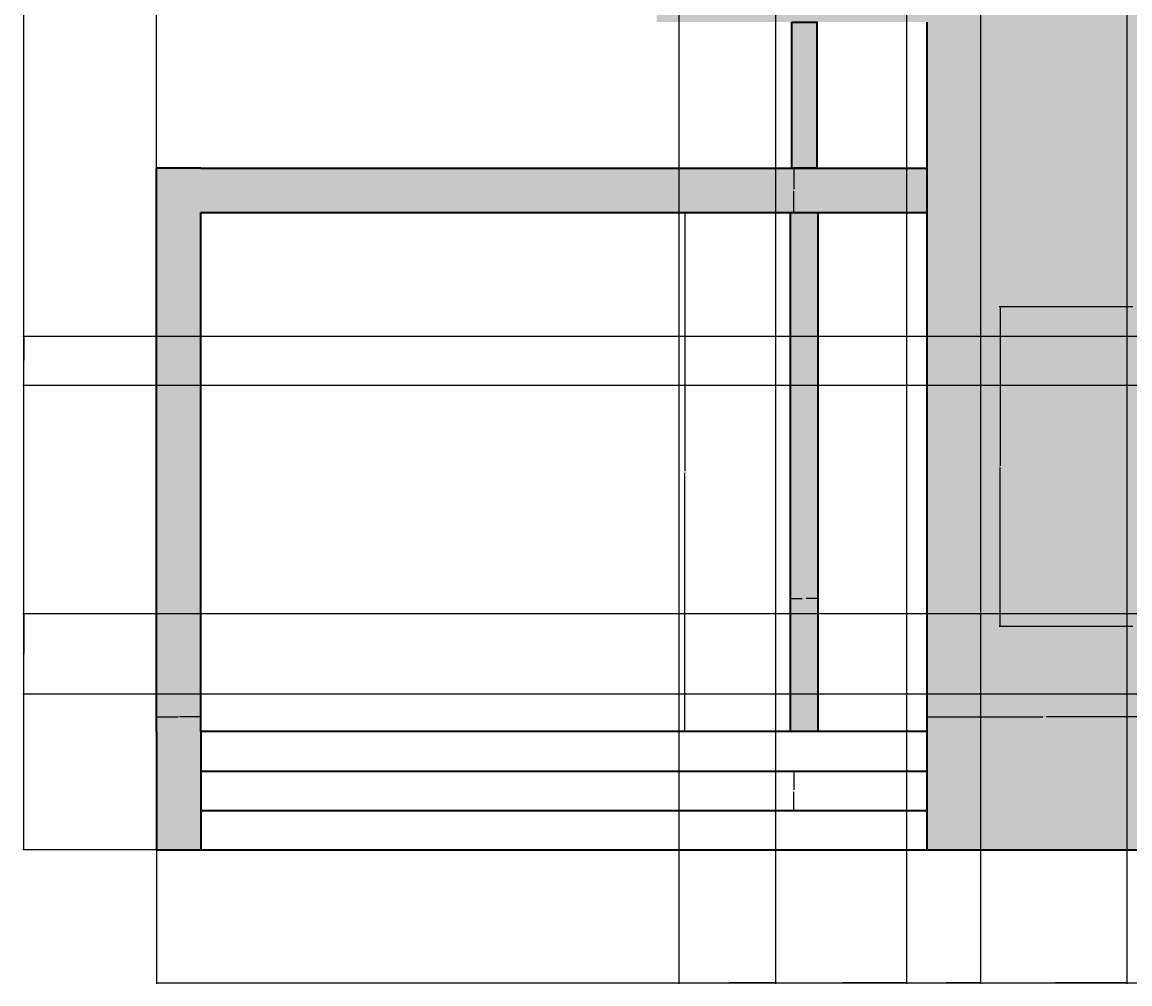
# Model space of a CAD drawing. Units: inches. Extents: x 73 to 607, y 92 to 651.
# Tile 1 of 18: x 73 to 298, y 116 to 311. Entities that reach past the tile are written whole.
import ezdxf

# ---------------------------------------------------------------- set-up
doc = ezdxf.new("R2010")
doc.units = ezdxf.units.IN
doc.header["$MEASUREMENT"] = 0
for name, color, linetype, lineweight in [('A-ANNO-DIMS', 2, 'Continuous', 18), ('A-ELEV', 7, 'Continuous', 35), ('A-ELEV-PATT-BKGD', 252, 'Continuous', 13), ('A-ELEV-PATT-SHAD', 8, 'Continuous', 13), ('A-ELEV-PATT-STON', 42, 'Continuous', 13), ('A-ELEV-PATT-WALL', 254, 'Continuous', 13)]:
    doc.layers.add(name, color=color, linetype=linetype, lineweight=lineweight)
doc.styles.get("Standard").update_dxf_attribs({"font": 'arial.ttf'})
doc.dimstyles.get("Standard").update_dxf_attribs({"dimtxt": 0.18, "dimasz": 0.18, "dimexe": 0.18, "dimexo": 0.0625, "dimgap": 0.09, "dimtad": 0, "dimtih": 1, "dimtoh": 1, "dimdec": 4, "dimzin": 0, "dimdsep": 46, "dimtxsty": 'Standard', "dimcen": 0.09, "dimadec": 0, "dimazin": 0, "dimtfac": 1, "dimtdec": 4, "dimtofl": 0, "dimtmove": 0, "dimatfit": 3, "dimfxl": 1, "dimtolj": 1, "dimtzin": 0, "dimarcsym": 0})

# ---------------------------------------------------------------- blocks, each defined once
blk = doc.blocks.new('*D4')
at = {"layer": 'A-ANNO-DIMS', "color": 0, "lineweight": -2, "transparency": 16777216}
for p, q in [((100.1, 143.14), (100.1, 116.02)), ((580.1, 143.14), (580.1, 116.02)), ((100.28, 116.2), (339.81, 116.2)), ((579.92, 116.2), (340.39, 116.2))]:
    blk.add_line(p, q, dxfattribs=at)
at = {"layer": 'A-ANNO-DIMS', "color": 0, "transparency": 16777216}
for points in [[(100.28, 116.23), (100.28, 116.17), (100.1, 116.2)], [(579.92, 116.23), (579.92, 116.17), (580.1, 116.2)]]:
    blk.add_solid(points, dxfattribs=at)
at = {"layer": 'Defpoints', "color": 0, "transparency": 16777216}
for p in [(100.1, 143.2), (580.1, 143.2), (580.1, 116.2)]:
    blk.add_point(p, dxfattribs=at)
at = {"layer": 'A-ANNO-DIMS', "color": 0, "transparency": 16777216, "insert": (340.1, 116.2), "char_height": 0.18, "attachment_point": 5}
blk.add_mtext('\\A1;480', dxfattribs=at)
blk = doc.blocks.new('*D5')
at = {"layer": 'A-ANNO-DIMS', "color": 0, "lineweight": -2, "transparency": 16777216}
for p, q in [((256.41, 623.8), (72.92, 623.8)), ((73.1, 623.62), (73.1, 383.68)), ((73.1, 143.38), (73.1, 383.32)), ((100.04, 143.2), (72.92, 143.2))]:
    blk.add_line(p, q, dxfattribs=at)
at = {"layer": 'A-ANNO-DIMS', "color": 0, "transparency": 16777216}
for points in [[(73.07, 623.62), (73.13, 623.62), (73.1, 623.8)], [(73.07, 143.38), (73.13, 143.38), (73.1, 143.2)]]:
    blk.add_solid(points, dxfattribs=at)
at = {"layer": 'Defpoints', "color": 0, "transparency": 16777216}
for p in [(73.1, 623.8), (256.47, 623.8), (100.1, 143.2)]:
    blk.add_point(p, dxfattribs=at)
at = {"layer": 'A-ANNO-DIMS', "color": 0, "transparency": 16777216, "insert": (73.1, 383.5), "char_height": 0.18, "attachment_point": 5}
blk.add_mtext('\\A1;480.6', dxfattribs=at)
blk = doc.blocks.new('*D6')
at = {"layer": 'A-ANNO-DIMS', "color": 0, "lineweight": -2, "transparency": 16777216}
for p, q in [((100.1, 281.67), (100.1, 650.98)), ((100.28, 650.8), (150.41, 650.8)), ((201.45, 650.8), (151.32, 650.8)), ((201.63, 412.7), (201.63, 650.98))]:
    blk.add_line(p, q, dxfattribs=at)
at = {"layer": 'A-ANNO-DIMS', "color": 0, "transparency": 16777216}
for points in [[(100.28, 650.83), (100.28, 650.77), (100.1, 650.8)], [(201.45, 650.83), (201.45, 650.77), (201.63, 650.8)]]:
    blk.add_solid(points, dxfattribs=at)
at = {"layer": 'Defpoints', "color": 0, "transparency": 16777216}
for p in [(201.63, 650.8), (201.63, 412.64), (100.1, 281.6)]:
    blk.add_point(p, dxfattribs=at)
at = {"layer": 'A-ANNO-DIMS', "color": 0, "transparency": 16777216, "insert": (150.87, 650.8), "char_height": 0.18, "attachment_point": 5}
blk.add_mtext('\\A1;101.54', dxfattribs=at)
blk = doc.blocks.new('*D26')
at = {"layer": 'A-ANNO-DIMS', "color": 0, "lineweight": -2, "transparency": 16777216}
for p, q in [((234.32, 272.6), (207.2, 272.6)), ((207.38, 272.42), (207.38, 220.09)), ((207.38, 167.38), (207.38, 219.72)), ((234.32, 167.2), (207.2, 167.2))]:
    blk.add_line(p, q, dxfattribs=at)
at = {"layer": 'A-ANNO-DIMS', "color": 0, "transparency": 16777216}
for points in [[(207.35, 272.42), (207.41, 272.42), (207.38, 272.6)], [(207.35, 167.38), (207.41, 167.38), (207.38, 167.2)]]:
    blk.add_solid(points, dxfattribs=at)
at = {"layer": 'Defpoints', "color": 0, "transparency": 16777216}
for p in [(207.38, 272.6), (234.38, 272.6), (234.38, 167.2)]:
    blk.add_point(p, dxfattribs=at)
at = {"layer": 'A-ANNO-DIMS', "color": 0, "transparency": 16777216, "insert": (207.38, 219.9), "char_height": 0.18, "attachment_point": 5}
blk.add_mtext('\\A1;105.4', dxfattribs=at)
blk = doc.blocks.new('*D27')
at = {"layer": 'A-ANNO-DIMS', "color": 0, "lineweight": -2, "transparency": 16777216}
for p, q in [((100.1, 143.27), (100.1, 170.38)), ((100.28, 170.2), (104.45, 170.2)), ((108.92, 170.2), (104.75, 170.2)), ((109.1, 143.27), (109.1, 170.38))]:
    blk.add_line(p, q, dxfattribs=at)
at = {"layer": 'A-ANNO-DIMS', "color": 0, "transparency": 16777216}
for points in [[(100.28, 170.23), (100.28, 170.17), (100.1, 170.2)], [(108.92, 170.23), (108.92, 170.17), (109.1, 170.2)]]:
    blk.add_solid(points, dxfattribs=at)
at = {"layer": 'Defpoints', "color": 0, "transparency": 16777216}
for p in [(109.1, 170.2), (100.1, 143.2), (109.1, 143.2)]:
    blk.add_point(p, dxfattribs=at)
at = {"layer": 'A-ANNO-DIMS', "color": 0, "transparency": 16777216, "insert": (104.6, 170.2), "char_height": 0.18, "attachment_point": 5}
blk.add_mtext('\\A1;9', dxfattribs=at)
blk = doc.blocks.new('*D28')
at = {"layer": 'A-ANNO-DIMS', "color": 0, "lineweight": -2, "transparency": 16777216}
for p, q in [((256.41, 281.6), (229.29, 281.6)), ((229.47, 281.42), (229.47, 277.29)), ((229.47, 272.78), (229.47, 276.92)), ((256.41, 272.6), (229.29, 272.6))]:
    blk.add_line(p, q, dxfattribs=at)
at = {"layer": 'A-ANNO-DIMS', "color": 0, "transparency": 16777216}
for points in [[(229.44, 281.42), (229.5, 281.42), (229.47, 281.6)], [(229.44, 272.78), (229.5, 272.78), (229.47, 272.6)]]:
    blk.add_solid(points, dxfattribs=at)
at = {"layer": 'Defpoints', "color": 0, "transparency": 16777216}
for p in [(229.47, 281.6), (256.47, 281.6), (256.47, 272.6)]:
    blk.add_point(p, dxfattribs=at)
at = {"layer": 'A-ANNO-DIMS', "color": 0, "transparency": 16777216, "insert": (229.47, 277.1), "char_height": 0.18, "attachment_point": 5}
blk.add_mtext('\\A1;9', dxfattribs=at)
blk = doc.blocks.new('*D29')
at = {"layer": 'A-ANNO-DIMS', "color": 0, "lineweight": -2, "transparency": 16777216}
for p, q in [((256.41, 159.2), (229.29, 159.2)), ((229.47, 159.02), (229.47, 155.39)), ((229.47, 151.38), (229.47, 155.02)), ((256.41, 151.2), (229.29, 151.2))]:
    blk.add_line(p, q, dxfattribs=at)
at = {"layer": 'A-ANNO-DIMS', "color": 0, "transparency": 16777216}
for points in [[(229.44, 159.02), (229.5, 159.02), (229.47, 159.2)], [(229.44, 151.38), (229.5, 151.38), (229.47, 151.2)]]:
    blk.add_solid(points, dxfattribs=at)
at = {"layer": 'Defpoints', "color": 0, "transparency": 16777216}
for p in [(229.47, 159.2), (256.47, 159.2), (256.47, 151.2)]:
    blk.add_point(p, dxfattribs=at)
at = {"layer": 'A-ANNO-DIMS', "color": 0, "transparency": 16777216, "insert": (229.47, 155.2), "char_height": 0.18, "attachment_point": 5}
blk.add_mtext('\\A1;8', dxfattribs=at)
blk = doc.blocks.new('*D30')
at = {"layer": 'A-ANNO-DIMS', "color": 0, "lineweight": -2, "transparency": 16777216}
for p, q in [((228.81, 167.27), (228.81, 194.38)), ((228.99, 194.2), (231.2, 194.2)), ((234.2, 194.2), (231.99, 194.2)), ((234.38, 167.27), (234.38, 194.38))]:
    blk.add_line(p, q, dxfattribs=at)
at = {"layer": 'A-ANNO-DIMS', "color": 0, "transparency": 16777216}
for points in [[(228.99, 194.23), (228.99, 194.17), (228.81, 194.2)], [(234.2, 194.23), (234.2, 194.17), (234.38, 194.2)]]:
    blk.add_solid(points, dxfattribs=at)
at = {"layer": 'Defpoints', "color": 0, "transparency": 16777216}
for p in [(234.38, 194.2), (228.81, 167.2), (234.38, 167.2)]:
    blk.add_point(p, dxfattribs=at)
at = {"layer": 'A-ANNO-DIMS', "color": 0, "transparency": 16777216, "insert": (231.6, 194.2), "char_height": 0.18, "attachment_point": 5}
blk.add_mtext('\\A1;5.576', dxfattribs=at)
blk = doc.blocks.new('*D31')
at = {"layer": 'A-ANNO-DIMS', "color": 0, "lineweight": -2, "transparency": 16777216}
for p, q in [((256.47, 143.27), (256.47, 170.38)), ((256.65, 170.2), (280.02, 170.2)), ((304.18, 170.2), (280.81, 170.2)), ((304.36, 143.27), (304.36, 170.38))]:
    blk.add_line(p, q, dxfattribs=at)
at = {"layer": 'A-ANNO-DIMS', "color": 0, "transparency": 16777216}
for points in [[(256.65, 170.23), (256.65, 170.17), (256.47, 170.2)], [(304.18, 170.23), (304.18, 170.17), (304.36, 170.2)]]:
    blk.add_solid(points, dxfattribs=at)
at = {"layer": 'Defpoints', "color": 0, "transparency": 16777216}
for p in [(304.36, 170.2), (256.47, 143.2), (304.36, 143.2)]:
    blk.add_point(p, dxfattribs=at)
at = {"layer": 'A-ANNO-DIMS', "color": 0, "transparency": 16777216, "insert": (280.41, 170.2), "char_height": 0.18, "attachment_point": 5}
blk.add_mtext('\\A1;47.88', dxfattribs=at)
blk = doc.blocks.new('*D34')
at = {"layer": 'A-ANNO-DIMS', "color": 0, "lineweight": -2, "transparency": 16777216}
for p, q in [((298.29, 253.41), (271.18, 253.41)), ((271.36, 253.23), (271.36, 221.16)), ((271.36, 188.73), (271.36, 220.79)), ((298.29, 188.55), (271.18, 188.55))]:
    blk.add_line(p, q, dxfattribs=at)
at = {"layer": 'A-ANNO-DIMS', "color": 0, "transparency": 16777216}
for points in [[(271.33, 253.23), (271.39, 253.23), (271.36, 253.41)], [(271.33, 188.73), (271.39, 188.73), (271.36, 188.55)]]:
    blk.add_solid(points, dxfattribs=at)
at = {"layer": 'Defpoints', "color": 0, "transparency": 16777216}
for p in [(271.36, 253.41), (298.36, 253.41), (298.36, 188.55)]:
    blk.add_point(p, dxfattribs=at)
at = {"layer": 'A-ANNO-DIMS', "color": 0, "transparency": 16777216, "insert": (271.36, 220.98), "char_height": 0.18, "attachment_point": 5}
blk.add_mtext('\\A1;64.86', dxfattribs=at)
blk = doc.blocks.new('*D73')
at = {"layer": 'A-ANNO-DIMS', "color": 0, "lineweight": -2, "transparency": 16777216}
for p, q in [((225.78, 347.13), (225.78, 116.02)), ((206.13, 320.14), (206.13, 116.02)), ((206.31, 116.2), (215.5, 116.2)), ((225.6, 116.2), (216.41, 116.2))]:
    blk.add_line(p, q, dxfattribs=at)
at = {"layer": 'A-ANNO-DIMS', "color": 0, "transparency": 16777216}
for points in [[(206.31, 116.23), (206.31, 116.17), (206.13, 116.2)], [(225.6, 116.23), (225.6, 116.17), (225.78, 116.2)]]:
    blk.add_solid(points, dxfattribs=at)
at = {"layer": 'Defpoints', "color": 0, "transparency": 16777216}
for p in [(225.78, 347.19), (206.13, 320.2), (225.78, 116.2)]:
    blk.add_point(p, dxfattribs=at)
at = {"layer": 'A-ANNO-DIMS', "color": 0, "transparency": 16777216, "insert": (215.96, 116.2), "char_height": 0.18, "attachment_point": 5}
blk.add_mtext('\\A1;19.645', dxfattribs=at)
blk = doc.blocks.new('*D74')
at = {"layer": 'A-ANNO-DIMS', "color": 0, "lineweight": -2, "transparency": 16777216}
for p, q in [((252.34, 363.04), (252.34, 116.02)), ((225.78, 347.13), (225.78, 116.02)), ((225.96, 116.2), (238.66, 116.2)), ((252.16, 116.2), (239.46, 116.2))]:
    blk.add_line(p, q, dxfattribs=at)
at = {"layer": 'A-ANNO-DIMS', "color": 0, "transparency": 16777216}
for points in [[(225.96, 116.23), (225.96, 116.17), (225.78, 116.2)], [(252.16, 116.23), (252.16, 116.17), (252.34, 116.2)]]:
    blk.add_solid(points, dxfattribs=at)
at = {"layer": 'Defpoints', "color": 0, "transparency": 16777216}
for p in [(252.34, 363.11), (225.78, 347.19), (252.34, 116.2)]:
    blk.add_point(p, dxfattribs=at)
at = {"layer": 'A-ANNO-DIMS', "color": 0, "transparency": 16777216, "insert": (239.06, 116.2), "char_height": 0.18, "attachment_point": 5}
blk.add_mtext('\\A1;26.56', dxfattribs=at)
blk = doc.blocks.new('*D75')
at = {"layer": 'A-ANNO-DIMS', "color": 0, "lineweight": -2, "transparency": 16777216}
for p, q in [((252.34, 363.04), (252.34, 116.02)), ((267.42, 345.14), (267.42, 116.02)), ((252.52, 116.2), (259.42, 116.2)), ((267.24, 116.2), (260.33, 116.2))]:
    blk.add_line(p, q, dxfattribs=at)
at = {"layer": 'A-ANNO-DIMS', "color": 0, "transparency": 16777216}
for points in [[(252.52, 116.23), (252.52, 116.17), (252.34, 116.2)], [(267.24, 116.23), (267.24, 116.17), (267.42, 116.2)]]:
    blk.add_solid(points, dxfattribs=at)
at = {"layer": 'Defpoints', "color": 0, "transparency": 16777216}
for p in [(252.34, 363.11), (267.42, 345.2), (267.42, 116.2)]:
    blk.add_point(p, dxfattribs=at)
at = {"layer": 'A-ANNO-DIMS', "color": 0, "transparency": 16777216, "insert": (259.88, 116.2), "char_height": 0.18, "attachment_point": 5}
blk.add_mtext('\\A1;15.074', dxfattribs=at)
blk = doc.blocks.new('*D76')
at = {"layer": 'A-ANNO-DIMS', "color": 0, "lineweight": -2, "transparency": 16777216}
for p, q in [((267.42, 345.14), (267.42, 116.02)), ((297.08, 334.98), (297.08, 116.02)), ((267.6, 116.2), (281.85, 116.2)), ((296.9, 116.2), (282.64, 116.2))]:
    blk.add_line(p, q, dxfattribs=at)
at = {"layer": 'A-ANNO-DIMS', "color": 0, "transparency": 16777216}
for points in [[(267.6, 116.23), (267.6, 116.17), (267.42, 116.2)], [(296.9, 116.23), (296.9, 116.17), (297.08, 116.2)]]:
    blk.add_solid(points, dxfattribs=at)
at = {"layer": 'Defpoints', "color": 0, "transparency": 16777216}
for p in [(267.42, 345.2), (297.08, 335.04), (297.08, 116.2)]:
    blk.add_point(p, dxfattribs=at)
at = {"layer": 'A-ANNO-DIMS', "color": 0, "transparency": 16777216, "insert": (282.25, 116.2), "char_height": 0.18, "attachment_point": 5}
blk.add_mtext('\\A1;29.66', dxfattribs=at)
blk = doc.blocks.new('*D92')
at = {"layer": 'A-ANNO-DIMS', "color": 0, "lineweight": -2, "transparency": 16777216}
for p, q in [((341.81, 247.41), (72.92, 247.41)), ((73.1, 247.23), (73.1, 242.61)), ((73.1, 237.63), (73.1, 242.25)), ((348.93, 237.45), (72.92, 237.45))]:
    blk.add_line(p, q, dxfattribs=at)
at = {"layer": 'A-ANNO-DIMS', "color": 0, "transparency": 16777216}
for points in [[(73.07, 247.23), (73.13, 247.23), (73.1, 247.41)], [(73.07, 237.63), (73.13, 237.63), (73.1, 237.45)]]:
    blk.add_solid(points, dxfattribs=at)
at = {"layer": 'Defpoints', "color": 0, "transparency": 16777216}
for p in [(341.87, 247.41), (73.1, 237.45), (349, 237.45)]:
    blk.add_point(p, dxfattribs=at)
at = {"layer": 'A-ANNO-DIMS', "color": 0, "transparency": 16777216, "insert": (73.1, 242.43), "char_height": 0.18, "attachment_point": 5}
blk.add_mtext('\\A1;9.95', dxfattribs=at)
blk = doc.blocks.new('*D119')
at = {"layer": 'A-ANNO-DIMS', "color": 0, "lineweight": -2, "transparency": 16777216}
for p, q in [((469.82, 191.14), (72.92, 191.14)), ((73.1, 190.96), (73.1, 183.15)), ((73.1, 174.98), (73.1, 182.79)), ((454.64, 174.8), (72.92, 174.8))]:
    blk.add_line(p, q, dxfattribs=at)
at = {"layer": 'A-ANNO-DIMS', "color": 0, "transparency": 16777216}
for points in [[(73.07, 190.96), (73.13, 190.96), (73.1, 191.14)], [(73.07, 174.98), (73.13, 174.98), (73.1, 174.8)]]:
    blk.add_solid(points, dxfattribs=at)
at = {"layer": 'Defpoints', "color": 0, "transparency": 16777216}
for p in [(73.1, 191.14), (469.88, 191.14), (454.7, 174.8)]:
    blk.add_point(p, dxfattribs=at)
at = {"layer": 'A-ANNO-DIMS', "color": 0, "transparency": 16777216, "insert": (73.1, 182.97), "char_height": 0.18, "attachment_point": 5}
blk.add_mtext('\\A1;16.34', dxfattribs=at)

msp = doc.modelspace()

# ---------------------------------------------------------------- hatches: boundary and pattern name
at = {"layer": 'A-ELEV-PATT-BKGD'}
h = msp.add_hatch(color=256, dxfattribs=at)
h.dxf.hatch_style = 1
h.paths.add_polyline_path([(321.3008, 479.2042), (312.3008, 479.2042), (312.3008, 478.7576), (312.3008, 412.636), (321.3008, 412.636)])
h.paths.add_polyline_path([(312.3008, 504.7576), (256.4726, 504.7576), (256.4726, 503.4576), (312.3008, 503.4576)], flags=17)
h.paths.add_polyline_path([(321.3008, 543.1576), (321.3008, 552.1576), (320.3257, 552.1576), (312.3008, 552.1576), (256.4726, 552.1576), (256.4726, 543.1576), (312.3008, 543.1576), (312.3008, 479.2042), (321.3008, 479.2042)])
h.paths.add_polyline_path([(451.5214, 412.636), (256.4726, 412.636), (256.4726, 403.636), (442.5214, 403.636), (442.5214, 320.2042), (206.1343, 320.2042), (206.1343, 320.9135), (206.1343, 403.636), (256.4726, 403.636), (256.4726, 412.636), (201.6343, 412.636), (201.6343, 320.9135), (201.6343, 320.2042), (201.6343, 311.2042), (256.4726, 311.2042), (451.5214, 311.2042)])
h.paths.add_polyline_path([(431.07, 258.6914), (369.5339, 258.6914), (369.5339, 247.4054), (396.692, 247.4054), (425.07, 247.4054), (425.07, 194.7312), (396.692, 194.6197), (396.692, 194.5366), (369.5339, 194.5366), (369.5339, 185.6619), (431.07, 185.6619)])
h.paths.add_polyline_path([(580.0983, 262.3024), (451.5214, 262.3024), (451.5214, 143.2042), (580.0983, 143.2042)])
h.paths.add_polyline_path([(454.7049, 174.802), (454.7049, 256.6321), (577.9249, 256.6321), (577.9249, 174.802)], flags=16)
h.paths.add_polyline_path([(465.9716, 191.1416, -1), (473.7874, 191.1416, -1)], flags=0)
h.paths.add_polyline_path([(490.5373, 181.6586, -1), (494.9999, 181.6586, -1)], flags=0)
h.paths.add_polyline_path([(476.2996, 209.8287, -1), (500.5844, 209.8287, -1)], flags=0)
h.paths.add_polyline_path([(505.3326, 194.7675, -1), (512.5843, 194.7675, -1)], flags=0)
h.paths.add_polyline_path([(520.9613, 186.679, -1), (526.544, 186.679, -1)], flags=0)
h.paths.add_polyline_path([(466.8103, 225.7267, -1), (470.1573, 225.7267, -1)], flags=0)
h.paths.add_polyline_path([(527.1059, 203.6926, -1), (536.0311, 203.6926, -1)], flags=0)
h.paths.add_polyline_path([(504.775, 232.6995, -1), (513.7002, 232.6995, -1)], flags=0)
h.paths.add_polyline_path([(546.9241, 183.611, -1), (554.7336, 183.611, -1)], flags=0)
h.paths.add_polyline_path([(459.5544, 243.856, -1), (466.8061, 243.856, -1)], flags=0)
h.paths.add_polyline_path([(476.3045, 246.924, -1), (488.5767, 246.924, -1)], flags=0)
h.paths.add_polyline_path([(529.9044, 226.8424, -1), (556.68, 226.8424, -1)], flags=0)
h.paths.add_polyline_path([(554.1814, 203.9716, -1), (561.4331, 203.9716, -1)], flags=0)
h.paths.add_polyline_path([(567.8561, 193.3729, -1), (570.6475, 193.3729, -1)], flags=0)
h.paths.add_polyline_path([(522.3584, 250.271, -1), (525.7053, 250.271, -1)], flags=0)
h.paths.add_polyline_path([(561.9965, 245.2506, -1), (567.5748, 245.2506, -1)], flags=0)
h.paths.add_polyline_path([(347.8686, 194.5366), (341.8686, 194.5366), (341.8686, 194.5452), (314.0144, 194.5452), (314.0144, 188.5452), (347.8686, 188.5452)])
h.paths.add_polyline_path([(347.8686, 253.4054), (314.0144, 253.4054), (314.0144, 247.4054), (341.8686, 247.4054), (347.8686, 247.4054)])
h.paths.add_polyline_path([(304.3559, 253.4054), (298.3559, 253.4054), (298.3559, 188.5452), (304.3559, 188.5452)])
h.paths.add_polyline_path([(450.6603, 552.1576), (369.9727, 552.1576), (369.9727, 479.2042), (374.4727, 479.2042), (374.4727, 547.6576), (446.1603, 547.6576), (446.1603, 479.2042), (450.6603, 479.2042)])
h.paths.add_polyline_path([(374.4727, 479.2042), (369.9727, 479.2042), (369.9727, 465.0632), (374.4727, 465.0632)])
h.paths.add_polyline_path([(450.6603, 479.2042), (446.1603, 479.2042), (446.1603, 465.0632), (450.6603, 465.0632)])
h.paths.add_polyline_path([(256.4726, 281.6039), (109.0983, 281.6039), (100.0983, 281.6039), (100.0983, 167.2042), (100.0983, 143.2042), (109.0983, 143.2042), (109.0983, 167.2042), (109.0983, 272.6039), (256.4726, 272.6039)])
at = {"layer": 'A-ELEV-PATT-SHAD'}
h = msp.add_hatch(color=256, dxfattribs=at)
h.dxf.hatch_style = 1
h.paths.add_polyline_path([(451.5214, 412.636), (256.4726, 412.636), (256.4726, 403.636), (442.5214, 403.636), (442.5214, 320.2042), (206.1343, 320.2042), (206.1343, 320.9135), (206.1343, 403.636), (256.4726, 403.636), (256.4726, 412.636), (201.6343, 412.636), (201.6343, 320.9135), (201.6343, 320.2042), (201.6343, 311.2042), (256.4726, 311.2042), (451.5214, 311.2042)])
h.paths.add_polyline_path([(580.0983, 262.3024), (451.5214, 262.3024), (451.5214, 143.2042), (580.0983, 143.2042)])
h.paths.add_polyline_path([(454.7049, 174.802), (454.7049, 256.6321), (577.9249, 256.6321), (577.9249, 174.802)], flags=16)
h.paths.add_polyline_path([(465.9716, 191.1416, -1), (473.7874, 191.1416, -1)], flags=0)
h.paths.add_polyline_path([(490.5373, 181.6586, -1), (494.9999, 181.6586, -1)], flags=0)
h.paths.add_polyline_path([(476.2996, 209.8287, -1), (500.5844, 209.8287, -1)], flags=0)
h.paths.add_polyline_path([(505.3326, 194.7675, -1), (512.5843, 194.7675, -1)], flags=0)
h.paths.add_polyline_path([(520.9613, 186.679, -1), (526.544, 186.679, -1)], flags=0)
h.paths.add_polyline_path([(466.8103, 225.7267, -1), (470.1573, 225.7267, -1)], flags=0)
h.paths.add_polyline_path([(527.1059, 203.6926, -1), (536.0311, 203.6926, -1)], flags=0)
h.paths.add_polyline_path([(459.5544, 243.856, -1), (466.8061, 243.856, -1)], flags=0)
h.paths.add_polyline_path([(504.775, 232.6995, -1), (513.7002, 232.6995, -1)], flags=0)
h.paths.add_polyline_path([(476.3045, 246.924, -1), (488.5767, 246.924, -1)], flags=0)
h.paths.add_polyline_path([(546.9241, 183.611, -1), (554.7336, 183.611, -1)], flags=0)
h.paths.add_polyline_path([(529.9044, 226.8424, -1), (556.68, 226.8424, -1)], flags=0)
h.paths.add_polyline_path([(554.1814, 203.9716, -1), (561.4331, 203.9716, -1)], flags=0)
h.paths.add_polyline_path([(522.3584, 250.271, -1), (525.7053, 250.271, -1)], flags=0)
h.paths.add_polyline_path([(567.8561, 193.3729, -1), (570.6475, 193.3729, -1)], flags=0)
h.paths.add_polyline_path([(561.9965, 245.2506, -1), (567.5748, 245.2506, -1)], flags=0)
h.paths.add_polyline_path([(431.07, 258.6914), (369.5339, 258.6914), (369.5339, 247.4054), (396.692, 247.4054), (425.07, 247.4054), (425.07, 194.7312), (396.692, 194.6197), (396.692, 194.5366), (369.5339, 194.5366), (369.5339, 185.6619), (431.07, 185.6619)])
h.paths.add_polyline_path([(347.8686, 253.4054), (314.0144, 253.4054), (314.0144, 247.4054), (341.8686, 247.4054), (347.8686, 247.4054)])
h.paths.add_polyline_path([(304.3559, 253.4054), (298.3559, 253.4054), (298.3559, 188.5452), (304.3559, 188.5452)])
h.paths.add_polyline_path([(347.8686, 194.5366), (341.8686, 194.5366), (341.8686, 194.5452), (314.0144, 194.5452), (314.0144, 188.5452), (347.8686, 188.5452)])
at = {"layer": 'A-ELEV-PATT-STON'}
h = msp.add_hatch(color=256, dxfattribs=at)
h.dxf.hatch_style = 1
h.paths.add_polyline_path([(394.7799, 623.801), (256.4726, 623.801), (256.4726, 586.3933), (394.7799, 586.3933)])
h.paths.add_polyline_path([(233.924, 582.9721), (229.3177, 582.9721), (229.3177, 412.636), (233.924, 412.636)])
h.paths.add_polyline_path([(234.1465, 311.2042), (229.0534, 311.2042), (229.0534, 281.6039), (234.1465, 281.6039)])
h.paths.add_polyline_path([(234.384, 272.6039), (228.8076, 272.6039), (228.8076, 167.2042), (234.384, 167.2042)])
at = {"layer": 'A-ELEV-PATT-WALL'}
h = msp.add_hatch(color=256, dxfattribs=at)
h.dxf.hatch_style = 1
h.paths.add_polyline_path([(509.9692, 483.857), (450.6603, 483.857), (450.6603, 465.0632), (446.1603, 465.0632), (446.1603, 484.2142), (374.4727, 484.2142), (374.4727, 465.0632), (369.9727, 465.0632), (369.9727, 484.2142), (321.3008, 484.2142), (321.3008, 412.636), (451.5214, 412.636), (451.5214, 311.2042), (314.0144, 311.2042), (314.0144, 253.4054), (347.8686, 253.4054), (347.8686, 247.4054), (369.5339, 247.4054), (369.5339, 258.6914), (431.07, 258.6914), (431.07, 185.6619), (369.5339, 185.6619), (369.5339, 194.5366), (347.8686, 194.5366), (347.8686, 188.5452), (314.0144, 188.5452), (314.0144, 143.2042), (451.5214, 143.2042), (451.5214, 262.3024), (580.0983, 262.3024), (580.0983, 311.2042), (509.9692, 311.2042)])
h.paths.add_polyline_path([(304.3559, 311.2042), (256.4726, 311.2042), (256.4726, 167.2042), (256.4726, 143.2042), (304.3559, 143.2042), (304.3559, 188.5452), (298.3559, 188.5452), (298.3559, 253.4054), (304.3559, 253.4054)])

# ---------------------------------------------------------------- linework, layer by layer
at = {"layer": 'A-ELEV'}
for p, q in [((256.4726, 311.2042), (256.4726, 167.2042)), ((100.0983, 167.2042), (100.0983, 281.6039)), ((109.0983, 281.6039), (100.0983, 281.6039)), ((109.0983, 281.6039), (256.4726, 281.6039)), ((109.0983, 167.2042), (109.0983, 272.6039)), ((109.0983, 272.6039), (256.4726, 272.6039)), ((100.0983, 167.2042), (100.0983, 143.2042)), ((109.0983, 167.2042), (109.0983, 143.2042)), ((256.4726, 167.2042), (109.0983, 167.2042)), ((256.4726, 167.2042), (256.4726, 143.2042)), ((109.0983, 159.2042), (256.4726, 159.2042)), ((109.0983, 151.2042), (256.4726, 151.2042)), ((100.0983, 143.2042), (580.0983, 143.2042))]:
    msp.add_line(p, q, dxfattribs=at)
for points in [[(229.0534, 311.2042), (234.1465, 311.2042), (234.1465, 281.6039), (229.0534, 281.6039)], [(228.8076, 272.6039), (234.384, 272.6039), (234.384, 167.2042), (228.8076, 167.2042)]]:
    msp.add_lwpolyline(points, close=True, dxfattribs=at)

# ---------------------------------------------------------------- dimensions: what is measured, and where the dimension line sits
at = {"layer": 'A-ANNO-DIMS'}
for base, p1, p2, override, picture, middle in [((201.6343, 650.801), (100.0983, 281.6039), (201.6343, 412.636), {"dimdec": 2, "dimlfac": 1, "dimrnd": 0, "dimzin": 0, "dimdsep": 46, "dimlunit": 2}, '*D6', (150.8663, 650.801)), ((252.3408, 116.2042), (225.7791, 347.1939), (252.3408, 363.1072), {"dimdec": 2, "dimlfac": 1, "dimrnd": 0, "dimzin": 0, "dimdsep": 46, "dimlunit": 2}, '*D74', (239.0599, 116.2042)), ((267.4151, 116.2042), (252.3408, 363.1072), (267.4151, 345.2025), {"dimdec": 3, "dimlfac": 1, "dimrnd": 0, "dimzin": 0, "dimdsep": 46, "dimlunit": 2}, '*D75', (259.878, 116.2042)), ((225.7791, 116.2042), (206.1343, 320.2042), (225.7791, 347.1939), {"dimdec": 3, "dimlfac": 1, "dimrnd": 0, "dimzin": 0, "dimdsep": 46, "dimlunit": 2}, '*D73', (215.9567, 116.2042)), ((297.0752, 116.2042), (267.4151, 345.2025), (297.0752, 335.0415), {"dimdec": 2, "dimlfac": 1, "dimrnd": 0, "dimzin": 0, "dimdsep": 46, "dimlunit": 2}, '*D76', (282.2451, 116.2042)), ((234.384, 194.2042), (228.8076, 167.2042), (234.384, 167.2042), {"dimdec": 3, "dimlfac": 1, "dimrnd": 0, "dimzin": 0, "dimdsep": 46, "dimlunit": 2}, '*D30', (231.5958, 194.2042)), ((109.0983, 170.2042), (100.0983, 143.2042), (109.0983, 143.2042), {"dimdec": 0, "dimlfac": 1, "dimrnd": 0, "dimzin": 0, "dimdsep": 46, "dimlunit": 2}, '*D27', (104.5983, 170.2042)), ((304.3559, 170.2042), (256.4726, 143.2042), (304.3559, 143.2042), {"dimdec": 2, "dimlfac": 1, "dimrnd": 0, "dimzin": 0, "dimdsep": 46, "dimlunit": 2}, '*D31', (280.4142, 170.2042)), ((580.0983, 116.2042), (100.0983, 143.2042), (580.0983, 143.2042), {"dimdec": 0, "dimlfac": 1, "dimrnd": 0, "dimzin": 0, "dimdsep": 46, "dimlunit": 2}, '*D4', (340.0983, 116.2042))]:
    dim = msp.add_linear_dim(base=base, p1=p1, p2=p2, dimstyle='Standard', override=override, dxfattribs=at)
    dim.commit()
    dim.dimension.update_dxf_attribs({"geometry": picture, "text_midpoint": middle})
for base, p1, p2, override, picture, middle in [((73.0983, 623.801), (100.0983, 143.2042), (256.4726, 623.801), {"dimdec": 1, "dimlfac": 1, "dimrnd": 0, "dimzin": 0, "dimdsep": 46, "dimlunit": 2}, '*D5', (73.0983, 383.5026)), ((229.4726, 281.6039), (256.4726, 272.6039), (256.4726, 281.6039), {"dimdec": 0, "dimlfac": 1, "dimrnd": 0, "dimzin": 0, "dimdsep": 46, "dimlunit": 2}, '*D28', (229.4726, 277.1039)), ((207.384, 272.6039), (234.384, 167.2042), (234.384, 272.6039), {"dimdec": 1, "dimlfac": 1, "dimrnd": 0, "dimzin": 0, "dimdsep": 46, "dimlunit": 2}, '*D26', (207.384, 219.9041)), ((271.3559, 253.4054), (298.3559, 188.5452), (298.3559, 253.4054), {"dimdec": 2, "dimlfac": 1, "dimrnd": 0, "dimzin": 0, "dimdsep": 46, "dimlunit": 2}, '*D34', (271.3559, 220.9753)), ((73.0983, 237.4546), (341.8686, 247.4054), (348.9968, 237.4546), {"dimdec": 2, "dimlfac": 1, "dimrnd": 0, "dimzin": 0, "dimdsep": 46, "dimlunit": 2}, '*D92', (73.0983, 242.43)), ((73.0983, 191.1416), (454.7049, 174.802), (469.8795, 191.1416), {"dimdec": 2, "dimlfac": 1, "dimrnd": 0, "dimzin": 0, "dimdsep": 46, "dimlunit": 2}, '*D119', (73.0983, 182.9718)), ((229.4726, 159.2042), (256.4726, 151.2042), (256.4726, 159.2042), {"dimdec": 0, "dimlfac": 1, "dimrnd": 0, "dimzin": 0, "dimdsep": 46, "dimlunit": 2}, '*D29', (229.4726, 155.2042))]:
    dim = msp.add_linear_dim(base=base, p1=p1, p2=p2, angle=90, dimstyle='Standard', override=override, dxfattribs=at)
    dim.commit()
    dim.dimension.update_dxf_attribs({"geometry": picture, "text_midpoint": middle})

doc.saveas('drawing.dxf')
